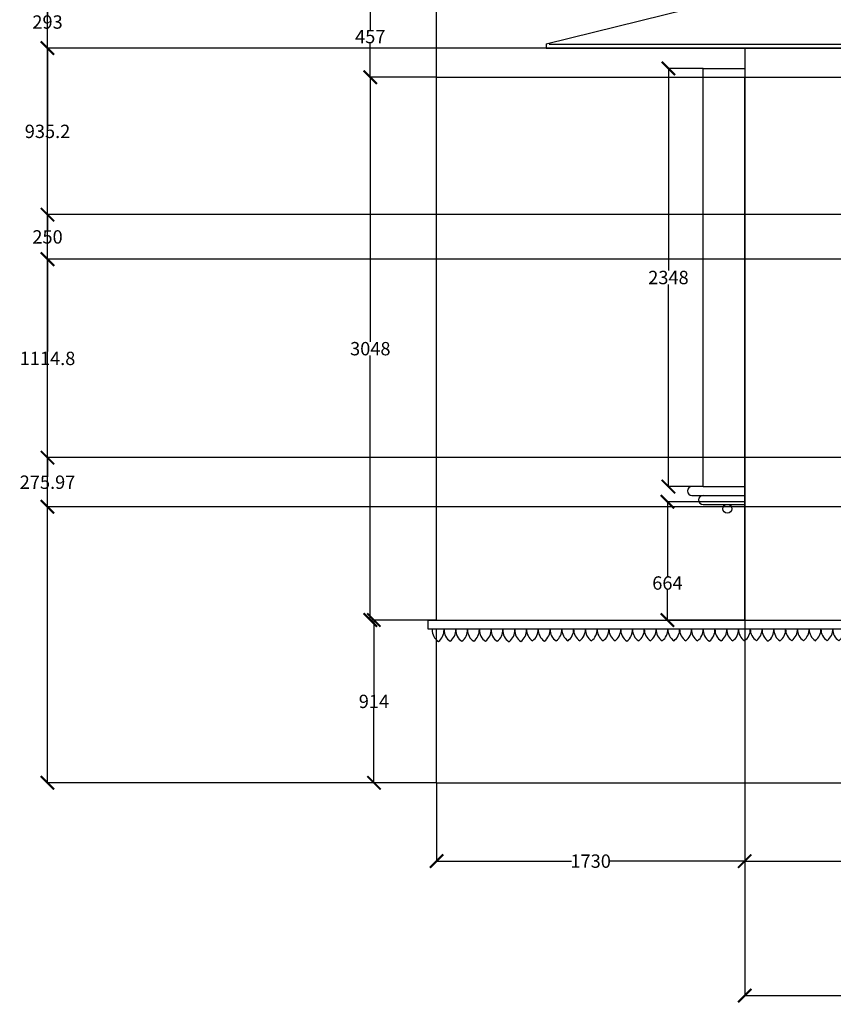
# Model space of a CAD drawing. Units: inches. Extents: x 829 to 33356404, y 1874 to 16983.
# Tile 1 of 9: x 829 to 5397, y 3502 to 9032. Entities that reach past the tile are written whole.
import ezdxf

# ---------------------------------------------------------------- set-up
doc = ezdxf.new("R2010")
doc.units = ezdxf.units.IN
doc.header["$MEASUREMENT"] = 0
doc.header["$PDMODE"] = 3
doc.layers.add('A-ANNO-DIMS', color=2, linetype='Continuous', lineweight=18)
doc.layers.add('A-ELEV', color=7, linetype='Continuous', lineweight=25)
doc.styles.get("Standard").update_dxf_attribs({"font": 'arial.ttf'})
doc.dimstyles.get("Standard").update_dxf_attribs({"dimtxt": 75, "dimasz": 75, "dimexe": 0.18, "dimexo": 0.0625, "dimgap": 0.09, "dimtad": 0, "dimtih": 1, "dimtoh": 1, "dimdec": 0, "dimzin": 0, "dimdsep": 46, "dimtxsty": 'Standard', "dimblk": 'ARCHTICK', "dimcen": 0.09, "dimadec": 0, "dimazin": 0, "dimtfac": 1, "dimtdec": 0, "dimtofl": 0, "dimtmove": 0, "dimatfit": 3, "dimfxl": 1, "dimtolj": 1, "dimtzin": 0, "dimarcsym": 0})

# ---------------------------------------------------------------- blocks, each defined once
blk = doc.blocks.new('_ArchTick')
at = {"color": 0, "linetype": 'ByBlock', "const_width": 0.15}
blk.add_lwpolyline([(-0.5, -0.5), (0.5, 0.5)], dxfattribs=at)
blk = doc.blocks.new('*D1')
at = {"layer": 'A-ANNO-DIMS', "color": 0, "lineweight": -2, "transparency": 16777216}
for p, q in [((3169.8, 4746.4), (3169.8, 4306.3)), ((4899.8, 4746.4), (4899.8, 4306.3)), ((3169.8, 4306.5), (3926.4, 4306.5)), ((4899.8, 4306.5), (4143.2, 4306.5))]:
    blk.add_line(p, q, dxfattribs=at)
at = {"layer": 'Defpoints', "color": 0, "transparency": 16777216}
for p in [(3169.8, 4746.5), (4899.8, 4746.5), (4899.8, 4306.5)]:
    blk.add_point(p, dxfattribs=at)
at = {"layer": 'A-ANNO-DIMS', "color": 0, "lineweight": -2, "transparency": 16777216, "xscale": 75, "yscale": 75, "zscale": 75, "rotation": 180}
blk.add_blockref('_ArchTick', (3169.8, 4306.5), dxfattribs=at)
at = {"layer": 'A-ANNO-DIMS', "color": 0, "lineweight": -2, "transparency": 16777216, "xscale": 75, "yscale": 75, "zscale": 75}
blk.add_blockref('_ArchTick', (4899.8, 4306.5), dxfattribs=at)
at = {"layer": 'A-ANNO-DIMS', "color": 0, "transparency": 16777216, "insert": (4034.8, 4306.5), "char_height": 75, "attachment_point": 5}
blk.add_mtext('\\A1;1730', dxfattribs=at)
blk = doc.blocks.new('*D2')
at = {"layer": 'A-ANNO-DIMS', "color": 0, "lineweight": -2, "transparency": 16777216}
for p, q in [((4899.8, 4746.4), (4899.8, 4306.1)), ((9559.8, 4711.5), (9559.8, 4306.1)), ((4899.8, 4306.3), (7116.3, 4306.3)), ((9559.8, 4306.3), (7343.2, 4306.3))]:
    blk.add_line(p, q, dxfattribs=at)
at = {"layer": 'Defpoints', "color": 0, "transparency": 16777216}
for p in [(4899.8, 4746.5), (9559.8, 4711.5), (9559.8, 4306.3)]:
    blk.add_point(p, dxfattribs=at)
at = {"layer": 'A-ANNO-DIMS', "color": 0, "lineweight": -2, "transparency": 16777216, "xscale": 75, "yscale": 75, "zscale": 75, "rotation": 180}
blk.add_blockref('_ArchTick', (4899.8, 4306.3), dxfattribs=at)
at = {"layer": 'A-ANNO-DIMS', "color": 0, "lineweight": -2, "transparency": 16777216, "xscale": 75, "yscale": 75, "zscale": 75}
blk.add_blockref('_ArchTick', (9559.8, 4306.3), dxfattribs=at)
at = {"layer": 'A-ANNO-DIMS', "color": 0, "transparency": 16777216, "insert": (7229.8, 4306.3), "char_height": 75, "attachment_point": 5}
blk.add_mtext('\\A1;4660', dxfattribs=at)
blk = doc.blocks.new('*D5')
at = {"layer": 'A-ANNO-DIMS', "color": 0, "lineweight": -2, "transparency": 16777216}
for p, q in [((3169.7, 8708.5), (2797.5, 8708.5)), ((2797.7, 8708.5), (2797.7, 7222.9)), ((2797.7, 5660.5), (2797.7, 7146.1)), ((3169.7, 5660.5), (2797.5, 5660.5))]:
    blk.add_line(p, q, dxfattribs=at)
at = {"layer": 'Defpoints', "color": 0, "transparency": 16777216}
for p in [(2797.7, 8708.5), (3169.8, 8708.5), (3169.8, 5660.5)]:
    blk.add_point(p, dxfattribs=at)
at = {"layer": 'A-ANNO-DIMS', "color": 0, "lineweight": -2, "transparency": 16777216, "xscale": 75, "yscale": 75, "zscale": 75}
for p, rotation in [((2797.7, 8708.5), 90), ((2797.7, 5660.5), 270)]:
    blk.add_blockref('_ArchTick', p, dxfattribs=dict(at, rotation=rotation))
at = {"layer": 'A-ANNO-DIMS', "color": 0, "transparency": 16777216, "insert": (2797.7, 7184.5), "char_height": 75, "attachment_point": 5}
blk.add_mtext('\\A1;3048', dxfattribs=at)
blk = doc.blocks.new('*D6')
at = {"layer": 'A-ANNO-DIMS', "color": 0, "lineweight": -2, "transparency": 16777216}
for p, q in [((3169.7, 5660.5), (2817.9, 5660.5)), ((2818.1, 5660.5), (2818.1, 5241.9)), ((2818.1, 4746.5), (2818.1, 5165.1)), ((3169.7, 4746.5), (2817.9, 4746.5))]:
    blk.add_line(p, q, dxfattribs=at)
at = {"layer": 'Defpoints', "color": 0, "transparency": 16777216}
for p in [(3169.8, 5660.5), (2818.1, 4746.5), (3169.8, 4746.5)]:
    blk.add_point(p, dxfattribs=at)
at = {"layer": 'A-ANNO-DIMS', "color": 0, "lineweight": -2, "transparency": 16777216, "xscale": 75, "yscale": 75, "zscale": 75}
for p, rotation in [((2818.1, 5660.5), 90), ((2818.1, 4746.5), 270)]:
    blk.add_blockref('_ArchTick', p, dxfattribs=dict(at, rotation=rotation))
at = {"layer": 'A-ANNO-DIMS', "color": 0, "transparency": 16777216, "insert": (2818.1, 5203.5), "char_height": 75, "attachment_point": 5}
blk.add_mtext('\\A1;914', dxfattribs=at)
blk = doc.blocks.new('*D7')
at = {"layer": 'A-ANNO-DIMS', "color": 0, "lineweight": -2, "transparency": 16777216}
for p, q in [((3169.7, 9165.5), (2797.3, 9165.5)), ((2797.5, 9165.5), (2797.5, 8975.2)), ((2797.5, 8708.5), (2797.5, 8898.7)), ((3169.7, 8708.5), (2797.3, 8708.5))]:
    blk.add_line(p, q, dxfattribs=at)
at = {"layer": 'Defpoints', "color": 0, "transparency": 16777216}
for p in [(3169.8, 9165.5), (2797.5, 8708.5), (3169.8, 8708.5)]:
    blk.add_point(p, dxfattribs=at)
at = {"layer": 'A-ANNO-DIMS', "color": 0, "lineweight": -2, "transparency": 16777216, "xscale": 75, "yscale": 75, "zscale": 75}
for p, rotation in [((2797.5, 9165.5), 90), ((2797.5, 8708.5), 270)]:
    blk.add_blockref('_ArchTick', p, dxfattribs=dict(at, rotation=rotation))
at = {"layer": 'A-ANNO-DIMS', "color": 0, "transparency": 16777216, "insert": (2797.5, 8937), "char_height": 75, "attachment_point": 5}
blk.add_mtext('\\A1;457', dxfattribs=at)
blk = doc.blocks.new('*D33')
at = {"layer": 'A-ANNO-DIMS', "color": 0, "lineweight": -2, "transparency": 16777216}
for p, q in [((4899.3, 6324.5), (4465.5, 6324.5)), ((4465.7, 6324.5), (4465.7, 5906.8)), ((4465.7, 5660.5), (4465.7, 5830)), ((4899.3, 5660.5), (4465.5, 5660.5))]:
    blk.add_line(p, q, dxfattribs=at)
at = {"layer": 'Defpoints', "color": 0, "transparency": 16777216}
for p in [(4465.7, 6324.5), (4899.4, 6324.5), (4899.4, 5660.5)]:
    blk.add_point(p, dxfattribs=at)
at = {"layer": 'A-ANNO-DIMS', "color": 0, "lineweight": -2, "transparency": 16777216, "xscale": 75, "yscale": 75, "zscale": 75}
for p, rotation in [((4465.7, 6324.5), 90), ((4465.7, 5660.5), 270)]:
    blk.add_blockref('_ArchTick', p, dxfattribs=dict(at, rotation=rotation))
at = {"layer": 'A-ANNO-DIMS', "color": 0, "transparency": 16777216, "insert": (4465.7, 5868.4), "char_height": 75, "attachment_point": 5}
blk.add_mtext('\\A1;664', dxfattribs=at)
blk = doc.blocks.new('*D39')
at = {"layer": 'A-ANNO-DIMS', "color": 0, "lineweight": -2, "transparency": 16777216}
for p, q in [((4665.8, 8758.2), (4471.2, 8758.2)), ((4471.4, 8758.2), (4471.4, 7622.6)), ((4471.4, 6410.2), (4471.4, 7545.8)), ((4665.8, 6410.2), (4471.2, 6410.2))]:
    blk.add_line(p, q, dxfattribs=at)
at = {"layer": 'Defpoints', "color": 0, "transparency": 16777216}
for p in [(4665.9, 8758.2), (4471.4, 6410.2), (4665.9, 6410.2)]:
    blk.add_point(p, dxfattribs=at)
at = {"layer": 'A-ANNO-DIMS', "color": 0, "lineweight": -2, "transparency": 16777216, "xscale": 75, "yscale": 75, "zscale": 75}
for p, rotation in [((4471.4, 8758.2), 90), ((4471.4, 6410.2), 270)]:
    blk.add_blockref('_ArchTick', p, dxfattribs=dict(at, rotation=rotation))
at = {"layer": 'A-ANNO-DIMS', "color": 0, "transparency": 16777216, "insert": (4471.4, 7584.2), "char_height": 75, "attachment_point": 5}
blk.add_mtext('\\A1;2348', dxfattribs=at)
blk = doc.blocks.new('*D83')
at = {"layer": 'A-ANNO-DIMS', "color": 0, "lineweight": -2, "transparency": 16777216}
for p, q in [((13604.5, 15734.9), (985.4, 15734.9)), ((985.6, 15734.9), (985.6, 10279.1)), ((985.6, 4746.5), (985.6, 10202.3)), ((3169.7, 4746.5), (985.4, 4746.5))]:
    blk.add_line(p, q, dxfattribs=at)
at = {"layer": 'Defpoints', "color": 0, "transparency": 16777216}
for p in [(985.6, 15734.9), (13604.5, 15734.9), (3169.8, 4746.5)]:
    blk.add_point(p, dxfattribs=at)
at = {"layer": 'A-ANNO-DIMS', "color": 0, "lineweight": -2, "transparency": 16777216, "xscale": 75, "yscale": 75, "zscale": 75}
for p, rotation in [((985.6, 15734.9), 90), ((985.6, 4746.5), 270)]:
    blk.add_blockref('_ArchTick', p, dxfattribs=dict(at, rotation=rotation))
at = {"layer": 'A-ANNO-DIMS', "color": 0, "transparency": 16777216, "insert": (985.6, 10240.7), "char_height": 75, "attachment_point": 5}
blk.add_mtext('\\A1;10988', dxfattribs=at)
blk = doc.blocks.new('*D86')
at = {"layer": 'A-ANNO-DIMS', "color": 0, "lineweight": -2, "transparency": 16777216}
for p, q in [((6385.6, 6424.4), (6385.6, 3551.3)), ((4900.3, 6410.1), (4900.3, 3551.3)), ((4900.3, 3551.5), (5490.7, 3551.5)), ((6385.6, 3551.5), (5795.2, 3551.5))]:
    blk.add_line(p, q, dxfattribs=at)
at = {"layer": 'Defpoints', "color": 0, "transparency": 16777216}
for p in [(6385.6, 6424.5), (4900.3, 6410.2), (6385.6, 3551.5)]:
    blk.add_point(p, dxfattribs=at)
at = {"layer": 'A-ANNO-DIMS', "color": 0, "lineweight": -2, "transparency": 16777216, "xscale": 75, "yscale": 75, "zscale": 75, "rotation": 180}
blk.add_blockref('_ArchTick', (4900.3, 3551.5), dxfattribs=at)
at = {"layer": 'A-ANNO-DIMS', "color": 0, "lineweight": -2, "transparency": 16777216, "xscale": 75, "yscale": 75, "zscale": 75}
blk.add_blockref('_ArchTick', (6385.6, 3551.5), dxfattribs=at)
at = {"layer": 'A-ANNO-DIMS', "color": 0, "transparency": 16777216, "insert": (5642.9, 3551.5), "char_height": 75, "attachment_point": 5}
blk.add_mtext('\\A1;1485.3', dxfattribs=at)
blk = doc.blocks.new('*D94')
at = {"layer": 'A-ANNO-DIMS', "color": 0, "lineweight": -2, "transparency": 16777216}
for p, q in [((9793.9, 6572.4), (985.4, 6572.4)), ((985.6, 6572.4), (985.6, 6472.8)), ((985.6, 6296.5), (985.6, 6396.1)), ((9559.7, 6296.5), (985.4, 6296.5))]:
    blk.add_line(p, q, dxfattribs=at)
at = {"layer": 'Defpoints', "color": 0, "transparency": 16777216}
for p in [(985.6, 6572.4), (9793.9, 6572.4), (9559.8, 6296.5)]:
    blk.add_point(p, dxfattribs=at)
at = {"layer": 'A-ANNO-DIMS', "color": 0, "lineweight": -2, "transparency": 16777216, "xscale": 75, "yscale": 75, "zscale": 75}
for p, rotation in [((985.6, 6572.4), 90), ((985.6, 6296.5), 270)]:
    blk.add_blockref('_ArchTick', p, dxfattribs=dict(at, rotation=rotation))
at = {"layer": 'A-ANNO-DIMS', "color": 0, "transparency": 16777216, "insert": (985.6, 6434.5), "char_height": 75, "attachment_point": 5}
blk.add_mtext('\\A1;275.97', dxfattribs=at)
blk = doc.blocks.new('*D95')
at = {"layer": 'A-ANNO-DIMS', "color": 0, "lineweight": -2, "transparency": 16777216}
for p, q in [((9793.9, 7687.3), (985.4, 7687.3)), ((985.6, 7687.3), (985.6, 7168.2)), ((985.6, 6572.4), (985.6, 7091.5)), ((9793.9, 6572.4), (985.4, 6572.4))]:
    blk.add_line(p, q, dxfattribs=at)
at = {"layer": 'Defpoints', "color": 0, "transparency": 16777216}
for p in [(985.6, 7687.3), (9793.9, 7687.3), (9793.9, 6572.4)]:
    blk.add_point(p, dxfattribs=at)
at = {"layer": 'A-ANNO-DIMS', "color": 0, "lineweight": -2, "transparency": 16777216, "xscale": 75, "yscale": 75, "zscale": 75}
for p, rotation in [((985.6, 7687.3), 90), ((985.6, 6572.4), 270)]:
    blk.add_blockref('_ArchTick', p, dxfattribs=dict(at, rotation=rotation))
at = {"layer": 'A-ANNO-DIMS', "color": 0, "transparency": 16777216, "insert": (985.6, 7129.8), "char_height": 75, "attachment_point": 5}
blk.add_mtext('\\A1;1114.8', dxfattribs=at)
blk = doc.blocks.new('*D96')
at = {"layer": 'A-ANNO-DIMS', "color": 0, "lineweight": -2, "transparency": 16777216}
for p, q in [((9793.7, 7937.3), (985.4, 7937.3)), ((985.6, 7937.3), (985.6, 7850.6)), ((985.6, 7687.3), (985.6, 7773.9)), ((9793.9, 7687.3), (985.4, 7687.3))]:
    blk.add_line(p, q, dxfattribs=at)
at = {"layer": 'Defpoints', "color": 0, "transparency": 16777216}
for p in [(985.6, 7937.3), (9793.7, 7937.3), (9793.9, 7687.3)]:
    blk.add_point(p, dxfattribs=at)
at = {"layer": 'A-ANNO-DIMS', "color": 0, "lineweight": -2, "transparency": 16777216, "xscale": 75, "yscale": 75, "zscale": 75}
for p, rotation in [((985.6, 7937.3), 90), ((985.6, 7687.3), 270)]:
    blk.add_blockref('_ArchTick', p, dxfattribs=dict(at, rotation=rotation))
at = {"layer": 'A-ANNO-DIMS', "color": 0, "transparency": 16777216, "insert": (985.6, 7812.3), "char_height": 75, "attachment_point": 5}
blk.add_mtext('\\A1;250', dxfattribs=at)
blk = doc.blocks.new('*D97')
at = {"layer": 'A-ANNO-DIMS', "color": 0, "lineweight": -2, "transparency": 16777216}
for p, q in [((9793.7, 8872.5), (985.4, 8872.5)), ((985.6, 8872.5), (985.6, 8443.3)), ((985.6, 7937.3), (985.6, 8366.5)), ((9793.7, 7937.3), (985.4, 7937.3))]:
    blk.add_line(p, q, dxfattribs=at)
at = {"layer": 'Defpoints', "color": 0, "transparency": 16777216}
for p in [(985.6, 8872.5), (9793.7, 8872.5), (9793.7, 7937.3)]:
    blk.add_point(p, dxfattribs=at)
at = {"layer": 'A-ANNO-DIMS', "color": 0, "lineweight": -2, "transparency": 16777216, "xscale": 75, "yscale": 75, "zscale": 75}
for p, rotation in [((985.6, 8872.5), 90), ((985.6, 7937.3), 270)]:
    blk.add_blockref('_ArchTick', p, dxfattribs=dict(at, rotation=rotation))
at = {"layer": 'A-ANNO-DIMS', "color": 0, "transparency": 16777216, "insert": (985.6, 8404.9), "char_height": 75, "attachment_point": 5}
blk.add_mtext('\\A1;935.2', dxfattribs=at)
blk = doc.blocks.new('*D98')
at = {"layer": 'A-ANNO-DIMS', "color": 0, "lineweight": -2, "transparency": 16777216}
for p, q in [((9793.7, 9165.5), (985.4, 9165.5)), ((985.6, 9165.5), (985.6, 9057.4)), ((985.6, 8872.5), (985.6, 8980.6)), ((9793.7, 8872.5), (985.4, 8872.5))]:
    blk.add_line(p, q, dxfattribs=at)
at = {"layer": 'Defpoints', "color": 0, "transparency": 16777216}
for p in [(985.6, 9165.5), (9793.7, 9165.5), (9793.7, 8872.5)]:
    blk.add_point(p, dxfattribs=at)
at = {"layer": 'A-ANNO-DIMS', "color": 0, "lineweight": -2, "transparency": 16777216, "xscale": 75, "yscale": 75, "zscale": 75}
for p, rotation in [((985.6, 9165.5), 90), ((985.6, 8872.5), 270)]:
    blk.add_blockref('_ArchTick', p, dxfattribs=dict(at, rotation=rotation))
at = {"layer": 'A-ANNO-DIMS', "color": 0, "transparency": 16777216, "insert": (985.6, 9019), "char_height": 75, "attachment_point": 5}
blk.add_mtext('\\A1;293', dxfattribs=at)

msp = doc.modelspace()

# ---------------------------------------------------------------- linework, layer by layer
at = {"layer": 'A-ELEV'}
for p, q in [((3169.778, 8708.468), (3169.778, 9165.468)), ((3784.24, 8897.468), (4872.426, 9165.468)), ((3784.24, 8897.468), (3784.24, 8872.468)), ((3784.24, 8872.468), (10626.905, 8872.468)), ((3802.555, 8894.205), (9793.728, 8897.385)), ((4899.383, 8872.468), (4899.383, 5610.468)), ((4665.878, 6410.159), (4665.878, 8758.159)), ((4665.878, 8758.159), (4899.383, 8758.159)), ((3169.778, 5660.468), (3169.778, 8708.468)), ((3169.778, 8708.468), (4900.278, 8708.468)), ((4900.278, 5660.468), (4900.278, 8708.468)), ((4900.278, 8708.468), (6385.56, 8708.468)), ((4665.878, 8590.899), (4665.878, 8590.899)), ((4603.091, 6360.159), (4900.278, 6360.159)), ((4665.878, 6410.159), (4900.278, 6410.159)), ((4665.878, 6310.159), (4900.278, 6310.159)), ((3119.778, 5660.468), (9559.893, 5660.468)), ((3119.778, 5660.468), (3119.778, 5610.468)), ((3119.778, 5610.468), (9559.887, 5610.468)), ((3169.778, 4746.468), (3169.778, 5610.468)), ((3169.778, 4746.468), (4899.778, 4746.468)), ((3169.778, 4746.468), (4899.778, 4746.468)), ((3169.778, 4746.468), (3329.778, 4746.468)), ((4899.778, 4746.468), (9559.778, 4746.468))]:
    msp.add_line(p, q, dxfattribs=at)
for points in [[(3145.469, 5605.68, 0.26781097), (3179.926, 5539.804, 0.24469844), (3211.558, 5605.68, 0.24469844)], [(3211.658, 5607.086, 0.26781097), (3246.115, 5541.21, 0.24469844), (3277.747, 5607.086, 0.24469844)], [(3277.659, 5607.08, 0.26781097), (3312.116, 5541.205, 0.24469844), (3343.748, 5607.08, 0.24469844)], [(3343.851, 5607.086, 0.26781097), (3378.309, 5541.21, 0.24469844), (3409.941, 5607.086, 0.24469844)], [(3409.941, 5607.086, 0.26781097), (3444.398, 5541.21, 0.24469844), (3476.03, 5607.086, 0.24469844)], [(3476.094, 5607.086, 0.26781097), (3510.551, 5541.21, 0.24469844), (3542.183, 5607.086, 0.24469844)], [(3542.224, 5607.086, 0.27512595), (3576.682, 5538.655, 0.25167024), (3608.314, 5607.086, 0.24469844)], [(3608.386, 5605.68, 0.26781097), (3642.843, 5539.804, 0.24469844), (3674.475, 5605.68, 0.24469844)], [(3674.639, 5610.166, 0.26781097), (3709.096, 5544.29, 0.24469844), (3740.728, 5610.166, 0.24469844)], [(3740.77, 5610.166, 0.27512595), (3775.227, 5541.734, 0.25167024), (3806.859, 5610.166, 0.24469844)], [(3806.931, 5608.759, 0.26781097), (3841.388, 5542.883, 0.24469844), (3873.02, 5608.759, 0.24469844)], [(3873.12, 5610.166, 0.26781097), (3907.578, 5544.29, 0.24469844), (3939.21, 5610.166, 0.24469844)], [(3939.121, 5610.16, 0.26781097), (3973.578, 5544.284, 0.24469844), (4005.21, 5610.16, 0.24469844)], [(4005.314, 5610.166, 0.26781097), (4039.771, 5544.29, 0.24469844), (4071.403, 5610.166, 0.24469844)], [(4071.403, 5610.166, 0.26781097), (4105.86, 5544.29, 0.24469844), (4137.492, 5610.166, 0.24469844)], [(4137.556, 5610.166, 0.26781097), (4172.013, 5544.29, 0.24469844), (4203.645, 5610.166, 0.24469844)], [(4203.687, 5610.166, 0.27512595), (4238.144, 5541.734, 0.25167024), (4269.776, 5610.166, 0.24469844)], [(4269.848, 5608.759, 0.26781097), (4304.305, 5542.883, 0.24469844), (4335.937, 5608.759, 0.24469844)], [(4336.038, 5610.166, 0.26781097), (4370.495, 5544.29, 0.24469844), (4402.127, 5610.166, 0.24469844)], [(4402.038, 5610.16, 0.26781097), (4436.495, 5544.284, 0.24469844), (4468.128, 5610.16, 0.24469844)], [(4468.231, 5610.166, 0.26781097), (4502.688, 5544.29, 0.24469844), (4534.32, 5610.166, 0.24469844)], [(4534.32, 5610.166, 0.26781097), (4568.777, 5544.29, 0.24469844), (4600.41, 5610.166, 0.24469844)], [(4600.41, 5610.166, 0.26781097), (4634.867, 5544.29, 0.24469844), (4666.499, 5610.166, 0.24469844)], [(4666.54, 5610.166, 0.27512595), (4700.997, 5541.734, 0.25167024), (4732.629, 5610.166, 0.24469844)], [(4732.702, 5608.759, 0.26781097), (4767.159, 5542.883, 0.24469844), (4798.791, 5608.759, 0.24469844)], [(4798.891, 5610.166, 0.26781097), (4833.348, 5544.29, 0.24469844), (4864.98, 5610.166, 0.24469844)], [(4864.892, 5610.16, 0.26781097), (4899.349, 5544.284, 0.24469844), (4930.981, 5610.16, 0.24469844)], [(4930.993, 5610.468, 0.26781097), (4965.45, 5544.592, 0.24469844), (4997.082, 5610.468, 0.24469844)], [(4997.124, 5610.468, 0.27512595), (5031.581, 5542.037, 0.25167024), (5063.213, 5610.468, 0.24469844)], [(5063.285, 5609.062, 0.26781097), (5097.742, 5543.186, 0.24469844), (5129.374, 5609.062, 0.24469844)], [(5129.475, 5610.468, 0.26781097), (5163.932, 5544.592, 0.24469844), (5195.564, 5610.468, 0.24469844)], [(5195.475, 5610.463, 0.26781097), (5229.932, 5544.587, 0.24469844), (5261.565, 5610.463, 0.24469844)], [(5261.668, 5610.468, 0.26781097), (5296.125, 5544.592, 0.24469844), (5327.757, 5610.468, 0.24469844)], [(5327.757, 5610.468, 0.26781097), (5362.214, 5544.592, 0.24469844), (5393.846, 5610.468, 0.24469844)], [(5393.91, 5610.468, 0.26781097), (5428.368, 5544.592, 0.24469844), (5460, 5610.468, 0.24469844)]]:
    msp.add_lwpolyline(points, format="xyb", dxfattribs=at)
msp.add_circle((4802.203, 6285.159), 25, dxfattribs=at)
for centre in [(4603.091, 6385.159), (4665.878, 6335.159)]:
    msp.add_arc(centre, 25, 90, 270, dxfattribs=at)

# ---------------------------------------------------------------- dimensions: what is measured, and where the dimension line sits
at = {"layer": 'A-ANNO-DIMS'}
for base, p1, p2, override, picture, middle in [((985.628, 15734.879), (3169.778, 4746.468), (13604.527, 15734.879), {"dimdec": 0, "dimlfac": 1, "dimrnd": 0, "dimzin": 0, "dimdsep": 46, "dimlunit": 2}, '*D83', (985.628, 10240.673)), ((985.628, 9165.468), (9793.728, 8872.468), (9793.728, 9165.468), {"dimdec": 0, "dimlfac": 1, "dimrnd": 0, "dimzin": 0, "dimdsep": 46, "dimlunit": 2}, '*D98', (985.628, 9018.968)), ((2797.522, 8708.468), (3169.778, 9165.468), (3169.778, 8708.468), {"dimclrd": 0, "dimclre": 0, "dimclrt": 0}, '*D7', (2797.522, 8936.968)), ((985.628, 8872.468), (9793.728, 7937.261), (9793.728, 8872.468), {"dimdec": 1, "dimlfac": 1, "dimrnd": 0, "dimzin": 0, "dimdsep": 46, "dimlunit": 2}, '*D97', (985.628, 8404.865)), ((4471.423, 6410.159), (4665.878, 8758.159), (4665.878, 6410.159), {"dimclrd": 0, "dimclre": 0, "dimclrt": 0}, '*D39', (4471.423, 7584.159)), ((2797.702, 8708.468), (3169.778, 5660.468), (3169.778, 8708.468), {"dimclrd": 0, "dimclre": 0, "dimclrt": 0}, '*D5', (2797.702, 7184.468)), ((985.628, 7937.261), (9793.914, 7687.262), (9793.728, 7937.261), {"dimdec": 0, "dimlfac": 1, "dimrnd": 0, "dimzin": 0, "dimdsep": 46, "dimlunit": 2}, '*D96', (985.628, 7812.261)), ((985.628, 7687.262), (9793.914, 6572.436), (9793.914, 7687.262), {"dimdec": 1, "dimlfac": 1, "dimrnd": 0, "dimzin": 0, "dimdsep": 46, "dimlunit": 2}, '*D95', (985.628, 7129.849)), ((985.628, 6572.436), (9559.804, 6296.468), (9793.914, 6572.436), {"dimdec": 2, "dimlfac": 1, "dimrnd": 0, "dimzin": 0, "dimdsep": 46, "dimlunit": 2}, '*D94', (985.628, 6434.452)), ((2818.088, 4746.468), (3169.778, 5660.468), (3169.778, 4746.468), {"dimclrd": 0, "dimclre": 0, "dimclrt": 0}, '*D6', (2818.088, 5203.468))]:
    dim = msp.add_linear_dim(base=base, p1=p1, p2=p2, angle=90, dimstyle='Standard', override=override, dxfattribs=at)
    dim.commit()
    dim.dimension.update_dxf_attribs({"geometry": picture, "text_midpoint": middle})
for base, p1, p2, override, picture, middle in [((6385.56, 3551.528), (4900.278, 6410.159), (6385.56, 6424.468), {"dimdec": 1, "dimlfac": 1, "dimrnd": 0, "dimzin": 0, "dimdsep": 46, "dimlunit": 2}, '*D86', (5642.919, 3551.528)), ((9559.778, 4306.306), (4899.778, 4746.468), (9559.778, 4711.528), {"dimclrd": 0, "dimclre": 0, "dimclrt": 0}, '*D2', (7229.778, 4306.306))]:
    dim = msp.add_linear_dim(base=base, p1=p1, p2=p2, dimstyle='Standard', override=override, dxfattribs=at)
    dim.commit()
    dim.dimension.update_dxf_attribs({"geometry": picture, "text_midpoint": middle})
dim = msp.add_linear_dim(base=(4465.683, 6324.468), p1=(4899.383, 5660.468), p2=(4899.383, 6324.468), angle=90, dimstyle='Standard', override={"dimclrd": 0, "dimclre": 0, "dimclrt": 0}, dxfattribs=at)
dim.commit()
dim.dimension.update_dxf_attribs({"geometry": '*D33', "text_midpoint": (4465.683, 5868.419), "dimtype": 160})
dim = msp.add_linear_dim(base=(4899.778, 4306.486), p1=(3169.778, 4746.468), p2=(4899.778, 4746.468), dimstyle='Standard', override={"dimclrd": 0, "dimclre": 0, "dimclrt": 0}, dxfattribs=at)
dim.commit()
dim.dimension.update_dxf_attribs({"geometry": '*D1', "text_midpoint": (4034.778, 4306.486), "dimtype": 160})

doc.saveas('drawing.dxf')
